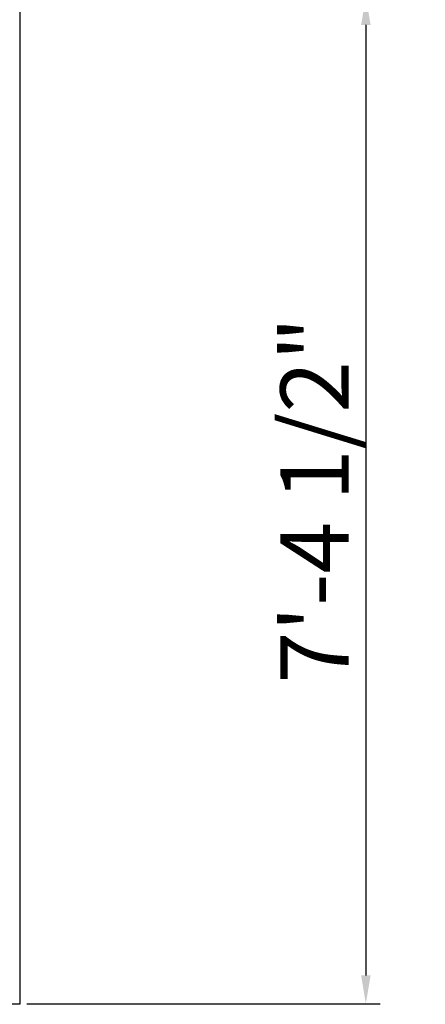
# Model space of a CAD drawing. Units: inches. Extents: x 459864 to 460310, y 324185 to 324787.
# Tile 78 of 112: x 460271 to 460307, y 324195 to 324281. Entities that reach past the tile are written whole.
import ezdxf

# ---------------------------------------------------------------- set-up
doc = ezdxf.new("R2010")
doc.units = ezdxf.units.IN
doc.layers.add('A-ANNO-DIMS', color=2, linetype='Continuous', lineweight=18)
doc.layers.add('C-PROP', color=7, linetype='Continuous', lineweight=30)
doc.styles.get("Standard").update_dxf_attribs({"font": 'arial.ttf'})
doc.dimstyles.new('ISO-25', dxfattribs={"dimtxt": 6, "dimasz": 2.5, "dimexe": 1.25, "dimexo": 0.625, "dimtad": 1, "dimdec": 1, "dimlunit": 3, "dimtxsty": 'Standard', "dimcen": 2.5, "dimadec": 0, "dimazin": 0, "dimtfac": 1, "dimtdec": 1, "dimtmove": 0, "dimatfit": 3, "dimfxl": 1, "dimarcsym": 0})

# ---------------------------------------------------------------- blocks, each defined once
blk = doc.blocks.new('*D65')
at = {"layer": 'A-ANNO-DIMS', "color": 0, "lineweight": -2, "transparency": 16777216}
for p, q in [((460247.74, 324283.483), (460302.765, 324283.483)), ((460301.515, 324280.983), (460301.515, 324197.483)), ((460271.74, 324194.983), (460302.765, 324194.983))]:
    blk.add_line(p, q, dxfattribs=at)
at = {"layer": 'A-ANNO-DIMS', "color": 0, "transparency": 16777216}
for points in [[(460301.098, 324280.983), (460301.932, 324280.983), (460301.515, 324283.483)], [(460301.098, 324197.483), (460301.932, 324197.483), (460301.515, 324194.983)]]:
    blk.add_solid(points, dxfattribs=at)
at = {"layer": 'Defpoints', "color": 0, "transparency": 16777216}
for p in [(460247.115, 324283.483), (460271.115, 324194.983), (460301.515, 324194.983)]:
    blk.add_point(p, dxfattribs=at)
at = {"layer": 'A-ANNO-DIMS', "color": 0, "transparency": 16777216, "insert": (460297.788, 324239.233), "char_height": 6, "attachment_point": 5, "rotation": 90}
blk.add_mtext('7\'-4 1/2"', dxfattribs=at)

msp = doc.modelspace()

# ---------------------------------------------------------------- linework, layer by layer
at = {"layer": 'C-PROP'}
for p, q in [((460271.115, 324466.483), (460271.115, 324194.947)), ((460061.115, 324194.983), (460271.115, 324194.983))]:
    msp.add_line(p, q, dxfattribs=at)

# ---------------------------------------------------------------- dimensions: what is measured, and where the dimension line sits
at = {"layer": 'A-ANNO-DIMS'}
dim = msp.add_linear_dim(base=(460301.515, 324194.983), p1=(460247.115, 324283.483), p2=(460271.115, 324194.983), angle=90, dimstyle='ISO-25', override={"dimdec": 1, "dimlfac": 1, "dimrnd": 0, "dimzin": 1, "dimdsep": 46, "dimlunit": 4, "dimfrac": 2}, dxfattribs=at)
dim.commit()
dim.dimension.update_dxf_attribs({"geometry": '*D65', "text_midpoint": (460297.788, 324239.233)})

doc.saveas('drawing.dxf')
